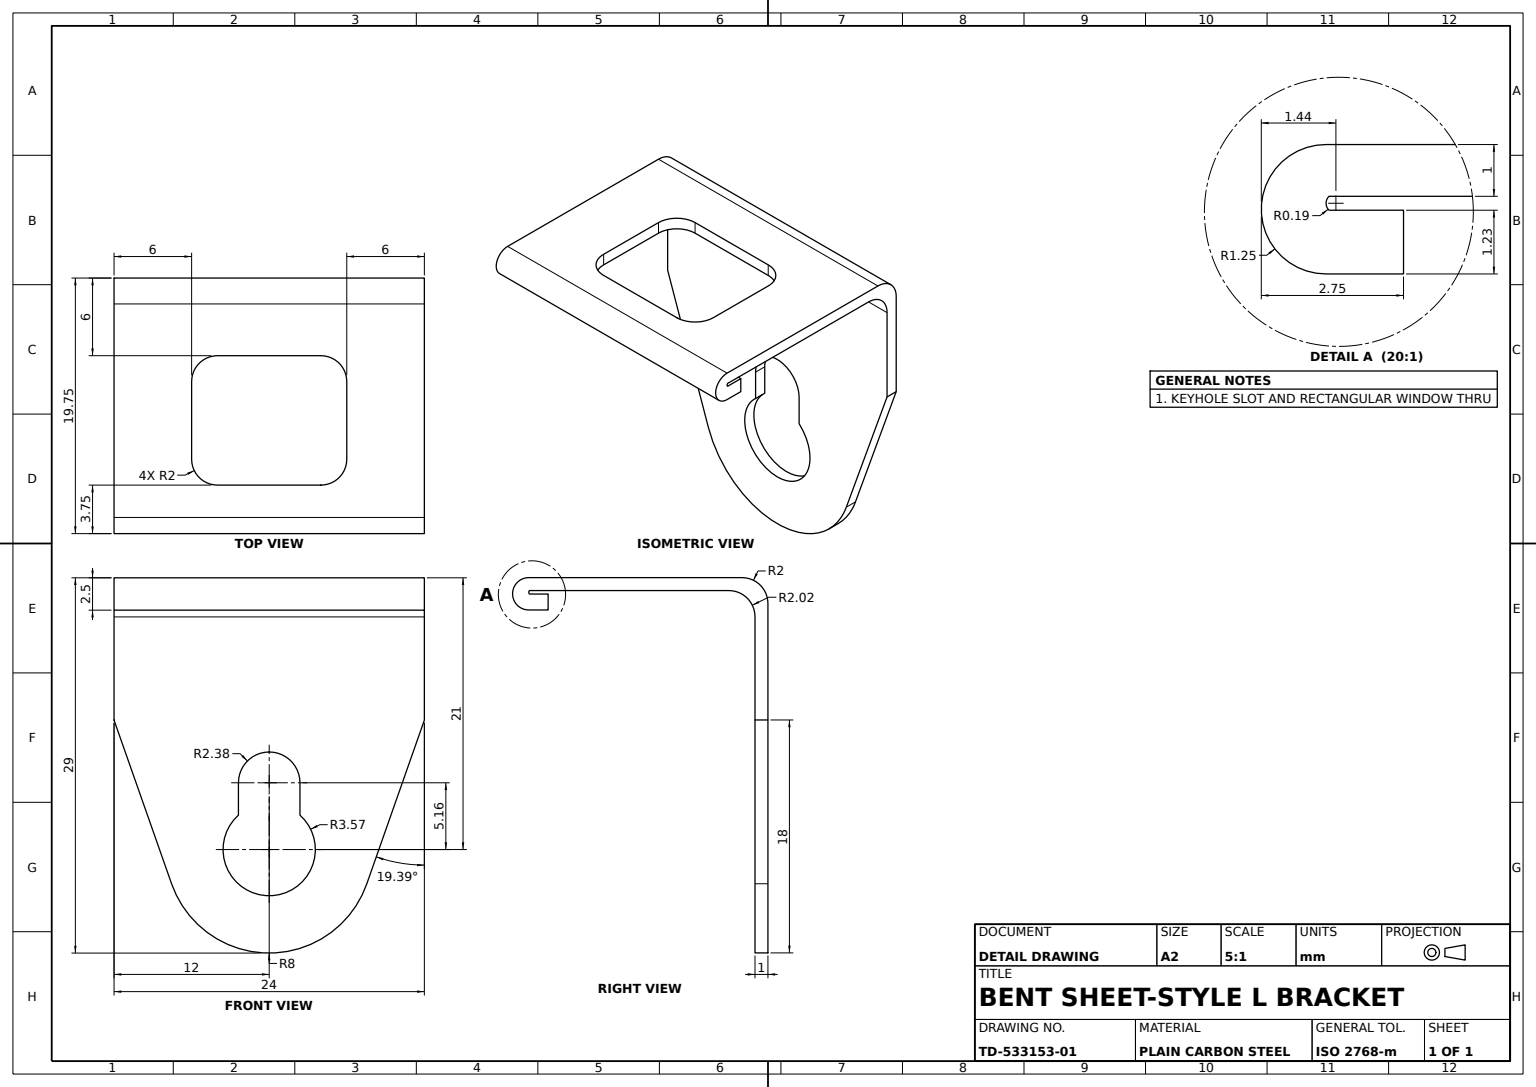
SolidWorks part; units mm, degrees
material "Plain Carbon Steel"
ref_plane "Front Plane" through (0, 0, 0) normal (0, 0, 1) x (1, 0, 0)
ref_plane "Top Plane" through (0, 0, 0) normal (0, 1, 0) x (1, 0, 0)
ref_plane "Right Plane" through (0, 0, 0) normal (1, 0, 0) x (0, 0, -1)
sketch "Bracket Profile Sketch" plane through (0, 0, 0) normal (0, 0, 1) x (1, 0, 0)
  line L0 (2, 0) -> (18.5, 0)
  line L1 (0, -2) -> (0, -29)
  line L2 (0, -29) -> (1, -29)
  line L3 (1, -29) -> (1, -3.0214)
  line L4 (3.0214, -1) -> (18.4416, -1)
  line L6 (18.5, -2.5) -> (18.5, 0) construction
  line L7 (18.4416, -1.2687) -> (17, -1.2687)
  line L8 (17, -2.5) -> (17, -1.2687)
  line L9 (18.5, -2.5) -> (17, -2.5)
  line L10 (18.4416, -1) -> (17, -1) construction
  line L11 (0, 0) -> (0, -33.6296) construction
  arc A0 (3.0214, -1) -> (1, -3.0214) centre (3.0214, -3.0214) ccw
  arc A1 (2, 0) -> (0, -2) centre (2, -2) ccw
  arc A2 (18.5, -2.5) -> (18.5, 0) centre (18.5, -1.25) ccw
  arc A3 (18.4416, -1) -> (18.4416, -1.2687) centre (18.3072, -1.1344) cw
  dimension "D1" = 18.5
  dimension "D3" = 1
  dimension "D4" = 2.5
  dimension "D6" = 2
  dimension "D7" = 29
  dimension "D9" = 0.19
  dimension "D2" = 16
  dimension "D5" = 1
  dimension "D8" = 25.9786
  dimension "D10" = 18.3072
  dimension "D11" = 1.2313
  dimension "D12" = 0.2248
  dimension "D13" = 13.9786
extrude "Bracket Body" add sketch "Bracket Profile Sketch" along normal mid plane 24
sketch "Rectangular Window Sketch" plane through (0, -1, 0) normal (0, -1, 0) x (1, 0, 0)
  line L0 (0, -12) -> (6.7623, -12) construction
  line L1 (3.0214, -12) -> (18.4416, -12) construction
  line L2 (6, 0) -> (6, 4) construction
  line L3 (16, 0) -> (16, 4) construction
  line L4 (6.7623, -12) -> (16.7623, -12) construction
  line L5 (8, -6) -> (14, -6)
  line L6 (6, -4) -> (6, 4)
  line L7 (8, 6) -> (14, 6)
  line L8 (16, 4) -> (16, -4)
  line L11 (6, 0) -> (16, 0) construction
  arc A0 (8, 6) -> (6, 4) centre (8, 4) ccw
  arc A2 (16, 4) -> (14, 6) centre (14, 4) ccw
  arc A3 (16, -4) -> (14, -6) centre (14, -4) cw
  arc A4 (8, -6) -> (6, -4) centre (8, -4) cw
  dimension "D1" = 2
  dimension "D5" = 2
  dimension "D2" = 6
  dimension "D3" = 6
  dimension "D4" = 10
  dimension "D6" = 6.7623
extrude "Rectangular Window Cut" cut sketch "Rectangular Window Sketch" against normal mid plane 10
sketch "Keyhole Slot Sketch" plane through (1, 0, 0) normal (1, 0, 0) x (0, 0, -1)
  line L0 (-12, -11) -> (-12, -29)
  line L1 (12, -29) -> (12, -3.0214) construction
  line L2 (0, 0) -> (0, -29) construction
  line L3 (-12, -29) -> (12, -29) construction
  line L4 (0, -29) -> (0, -21) construction
  line L5 (12, -11) -> (7.5464, -23.6556)
  line L6 (-12, -11) -> (-7.5464, -23.6556)
  line L7 (-12, -29) -> (12, -29)
  line L8 (12, -29) -> (12, -11)
  arc A0 (-7.5464, -23.6556) -> (7.5464, -23.6556) centre (0, -21) ccw
  line M8 (12, -29) -> (12, -3.0214)
  line M10 (-12, -3.0214) -> (-12, -29)
  line M11 (-12, -29) -> (12, -29)
  dimension "D1" = 8
  dimension "D2" = 12.6556
extrude "Keyhole Slot Cut" cut sketch "Keyhole Slot Sketch" against normal blind 10 contours A0 L7 L5 M8 | A0 L6 M10 M11
sketch "Edge Notch Sketch" plane through (1, 0, 0) normal (1, 0, 0) x (0, 0, -1)
  line L0 (12, 0) -> (12, -15.84) construction
  line L1 (12, -15.84) -> (0, -15.84) construction
  line L2 (0, -15.84) -> (0, -21) construction
  line L3 (-2.38, -15.84) -> (-2.38, -18.3391)
  line L4 (2.38, -15.84) -> (2.38, -18.3391)
  arc A0 (2.38, -15.84) -> (-2.38, -15.84) centre (0, -15.84) ccw
  arc A1 (-2.38, -18.3391) -> (2.38, -18.3391) centre (0, -21) ccw
  dimension "D1" = 15.84
  dimension "D2" = 2.38
  dimension "D3" = 3.57
  dimension "D4" = 5.16
extrude "Edge Notch Cut" cut sketch "Edge Notch Sketch" against normal blind 2
